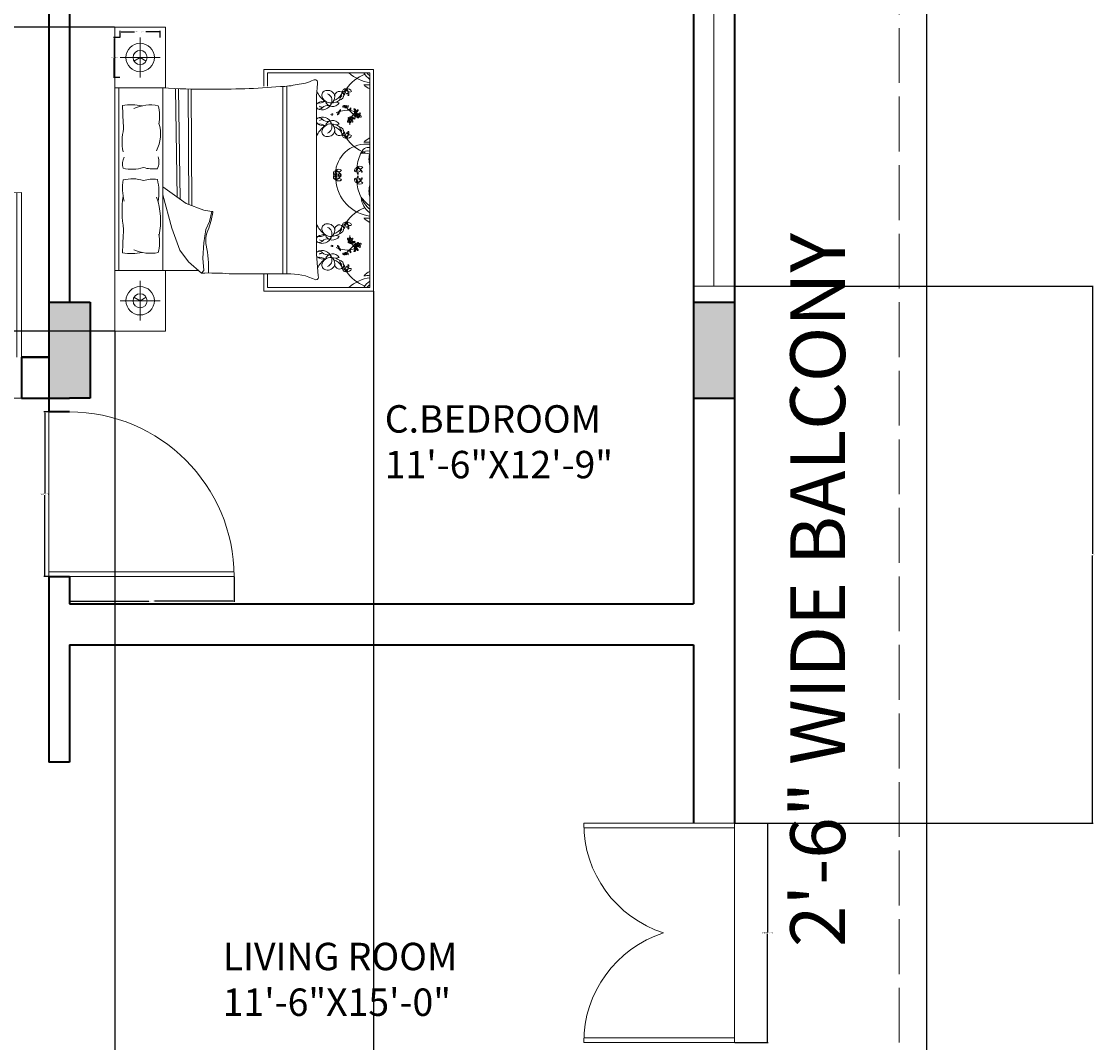
# Model space of a CAD drawing. Units: inches. Extents: x -36 to 401, y -686 to 73.
# Tile 14 of 15: x 167 to 401, y -319 to -96. Entities that reach past the tile are written whole.
import ezdxf

# ---------------------------------------------------------------- set-up
doc = ezdxf.new("R2010")
doc.units = ezdxf.units.IN
doc.header["$MEASUREMENT"] = 0
doc.linetypes.add('ACAD_ISO02W100', pattern=[15, 12, -3])
for name, color, linetype, lineweight in [('A-ANNO-DIMS', 2, 'Continuous', 18), ('A-AREA-IDEN', 7, 'Continuous', 18), ('A-COLS', 7, 'Continuous', 40), ('A-COLS-PATT', 22, 'Continuous', 13), ('A-DOOR', 3, 'Continuous', 18), ('A-FLOR-OVHD', 8, 'ACAD_ISO02W100', 18), ('A-FURN', 8, 'Continuous', 13), ('A-GLAZ', 4, 'Continuous', 18), ('A-WALL', 7, 'Continuous', 35), ('C-PROP', 7, 'Continuous', 25)]:
    doc.layers.add(name, color=color, linetype=linetype, lineweight=lineweight)
doc.styles.get("Standard").update_dxf_attribs({"font": 'arial.ttf'})
doc.dimstyles.get("Standard").update_dxf_attribs({"dimtxt": 0.18, "dimasz": 0.18, "dimexe": 0.18, "dimexo": 0.0625, "dimgap": 0.09, "dimtad": 0, "dimtih": 1, "dimtoh": 1, "dimdec": 0, "dimzin": 0, "dimdsep": 46, "dimlunit": 3, "dimtxsty": 'Standard', "dimcen": 0.09, "dimadec": 0, "dimazin": 0, "dimtfac": 1, "dimtdec": 0, "dimtofl": 0, "dimtmove": 0, "dimatfit": 3, "dimfxl": 1, "dimtolj": 1, "dimtzin": 0, "dimarcsym": 0})

# ---------------------------------------------------------------- blocks, each defined once
blk = doc.blocks.new('WIN-60IN')
for p, q in [((0, 9), (60, 9)), ((0, 0), (0, 9)), ((60, 9), (60, 0)), ((0, 4.5), (60, 4.5)), ((60, 0), (0, 0))]:
    blk.add_line(p, q)
blk = doc.blocks.new('DOOR-SWING-36IN')
for p, q in [((-1, 0), (-1, 36)), ((0, 0), (0, 36))]:
    blk.add_line(p, q)
blk.add_arc((0, 0), 36, 90, 180)
blk = doc.blocks.new('DOOR-PAIR-48IN')
for p, q in [((0, 48), (-24, 48)), ((0, 47), (-24, 47)), ((9, 48), (0, 48)), ((9, 47), (0, 47)), ((0, 1), (-24, 1)), ((0, 0), (-24, 0)), ((0, 1), (9, 1)), ((0, 0), (9, 0))]:
    blk.add_line(p, q)
for centre, start, end in [((1.23, 48), 180, 252.0547), ((1.23, 0), 107.9453, 180)]:
    blk.add_arc(centre, 25.23, start, end)
blk = doc.blocks.new('LAMP-BEDSIDE-SMALL')
for p, q in [((4.35, 0), (4.35, 8.7)), ((8.7, 4.35), (0, 4.35))]:
    blk.add_line(p, q)
for points in [[(4.35, 4.35), (3, 3.57)], [(4.35, 4.35), (5.69, 3.57)]]:
    blk.add_lwpolyline(points)
for radius in [3.11, 1.55]:
    blk.add_circle((4.35, 4.35), radius)
blk = doc.blocks.new('*D41')
at = {"layer": 'A-ANNO-DIMS', "color": 0, "lineweight": -2, "transparency": 16777216}
for p, q in [((177.13, -181.21), (171.61, -181.21)), ((171.79, -181.39), (171.79, -199.03)), ((171.79, -217.03), (171.79, -199.39)), ((177.13, -217.21), (171.61, -217.21))]:
    blk.add_line(p, q, dxfattribs=at)
at = {"layer": 'A-ANNO-DIMS', "color": 0, "transparency": 16777216}
for points in [[(171.76, -181.39), (171.82, -181.39), (171.79, -181.21)], [(171.76, -217.03), (171.82, -217.03), (171.79, -217.21)]]:
    blk.add_solid(points, dxfattribs=at)
at = {"layer": 'Defpoints', "color": 0, "transparency": 16777216}
for p in [(177.19, -181.21), (171.79, -217.21), (177.19, -217.21)]:
    blk.add_point(p, dxfattribs=at)
at = {"layer": 'A-ANNO-DIMS', "color": 0, "transparency": 16777216, "insert": (171.79, -199.21), "char_height": 0.18, "attachment_point": 5}
blk.add_mtext('\\A1;DOOR 3\'-0" TYP.', dxfattribs=at)
blk = doc.blocks.new('*D42')
at = {"layer": 'A-ANNO-DIMS', "color": 0, "lineweight": -2, "transparency": 16777216}
for p, q in [((177.19, -217.27), (177.19, -222.79)), ((213.19, -217.27), (213.19, -222.79)), ((177.37, -222.61), (194.55, -222.61)), ((213.01, -222.61), (195.83, -222.61))]:
    blk.add_line(p, q, dxfattribs=at)
at = {"layer": 'A-ANNO-DIMS', "color": 0, "transparency": 16777216}
for points in [[(177.37, -222.58), (177.37, -222.64), (177.19, -222.61)], [(213.01, -222.58), (213.01, -222.64), (213.19, -222.61)]]:
    blk.add_solid(points, dxfattribs=at)
at = {"layer": 'Defpoints', "color": 0, "transparency": 16777216}
for p in [(177.19, -217.21), (213.19, -217.21), (213.19, -222.61)]:
    blk.add_point(p, dxfattribs=at)
at = {"layer": 'A-ANNO-DIMS', "color": 0, "transparency": 16777216, "insert": (195.19, -222.61), "char_height": 0.18, "attachment_point": 5}
blk.add_mtext('\\A1;3\'-0" TYP.', dxfattribs=at)
blk = doc.blocks.new('*D45')
at = {"layer": 'A-ANNO-DIMS', "color": 0, "lineweight": -2, "transparency": 16777216}
for p, q in [((322.75, -271.21), (330.07, -271.21)), ((329.89, -271.39), (329.89, -295.03)), ((329.89, -319.03), (329.89, -295.39)), ((322.75, -319.21), (330.07, -319.21))]:
    blk.add_line(p, q, dxfattribs=at)
at = {"layer": 'A-ANNO-DIMS', "color": 0, "transparency": 16777216}
for points in [[(329.86, -271.39), (329.92, -271.39), (329.89, -271.21)], [(329.86, -319.03), (329.92, -319.03), (329.89, -319.21)]]:
    blk.add_solid(points, dxfattribs=at)
at = {"layer": 'Defpoints', "color": 0, "transparency": 16777216}
for p in [(322.69, -271.21), (329.89, -271.21), (322.69, -319.21)]:
    blk.add_point(p, dxfattribs=at)
at = {"layer": 'A-ANNO-DIMS', "color": 0, "transparency": 16777216, "insert": (329.89, -295.21), "char_height": 0.18, "attachment_point": 5}
blk.add_mtext('\\A1;DOOR PAIR 4\'-0" TYP.', dxfattribs=at)
blk = doc.blocks.new('*D59')
at = {"layer": 'A-ANNO-DIMS', "color": 0, "lineweight": -2, "transparency": 16777216}
for p, q in [((188.3, -99.23), (188.3, -97.81)), ((188.48, -97.99), (191.43, -97.99)), ((196.82, -97.99), (193.87, -97.99)), ((197, -99.23), (197, -97.81))]:
    blk.add_line(p, q, dxfattribs=at)
at = {"layer": 'A-ANNO-DIMS', "color": 0, "transparency": 16777216}
for points in [[(188.48, -97.96), (188.48, -98.02), (188.3, -97.99)], [(196.82, -97.96), (196.82, -98.02), (197, -97.99)]]:
    blk.add_solid(points, dxfattribs=at)
at = {"layer": 'Defpoints', "color": 0, "transparency": 16777216}
for p in [(197, -97.99), (188.3, -99.29), (197, -99.29)]:
    blk.add_point(p, dxfattribs=at)
at = {"layer": 'A-ANNO-DIMS', "color": 0, "transparency": 16777216, "insert": (192.65, -97.99), "char_height": 0.18, "attachment_point": 5}
blk.add_mtext('\\A1;LAMP 0\'-8 1/2" TYP.', dxfattribs=at)
blk = doc.blocks.new('*D60')
at = {"layer": 'A-ANNO-DIMS', "color": 0, "lineweight": -2, "transparency": 16777216}
for p, q in [((188.24, -99.29), (186.82, -99.29)), ((187, -99.47), (187, -103.46)), ((187, -107.81), (187, -103.82)), ((188.24, -107.99), (186.82, -107.99))]:
    blk.add_line(p, q, dxfattribs=at)
at = {"layer": 'A-ANNO-DIMS', "color": 0, "transparency": 16777216}
for points in [[(186.97, -99.47), (187.03, -99.47), (187, -99.29)], [(186.97, -107.81), (187.03, -107.81), (187, -107.99)]]:
    blk.add_solid(points, dxfattribs=at)
at = {"layer": 'Defpoints', "color": 0, "transparency": 16777216}
for p in [(187, -99.29), (188.3, -99.29), (188.3, -107.99)]:
    blk.add_point(p, dxfattribs=at)
at = {"layer": 'A-ANNO-DIMS', "color": 0, "transparency": 16777216, "insert": (187, -103.64), "char_height": 0.18, "attachment_point": 5}
blk.add_mtext('\\A1;0\'-8 1/2" TYP.', dxfattribs=at)
blk = doc.blocks.new('*D71')
at = {"layer": 'A-ANNO-DIMS', "color": 0, "lineweight": -2, "transparency": 16777216}
for p, q in [((322.75, -153.68), (401.17, -153.68)), ((400.99, -153.86), (400.99, -212.26)), ((400.99, -271.03), (400.99, -212.63)), ((322.75, -271.21), (401.17, -271.21))]:
    blk.add_line(p, q, dxfattribs=at)
at = {"layer": 'A-ANNO-DIMS', "color": 0, "transparency": 16777216}
for points in [[(400.96, -153.86), (401.02, -153.86), (400.99, -153.68)], [(400.96, -271.03), (401.02, -271.03), (400.99, -271.21)]]:
    blk.add_solid(points, dxfattribs=at)
at = {"layer": 'Defpoints', "color": 0, "transparency": 16777216}
for p in [(322.69, -153.68), (322.69, -271.21), (400.99, -271.21)]:
    blk.add_point(p, dxfattribs=at)
at = {"layer": 'A-ANNO-DIMS', "color": 0, "transparency": 16777216, "insert": (400.99, -212.44), "char_height": 0.18, "attachment_point": 5}
blk.add_mtext('\\A1;9\'-9 1/2"', dxfattribs=at)
blk = doc.blocks.new('*D87')
at = {"layer": 'A-ANNO-DIMS', "color": 0, "lineweight": -2, "transparency": 16777216}
for p, q in [((243.7, -154.81), (243.7, -685.69)), ((187.11, -163.6), (187.11, -685.69)), ((187.29, -685.51), (214.86, -685.51)), ((243.52, -685.51), (215.95, -685.51))]:
    blk.add_line(p, q, dxfattribs=at)
at = {"layer": 'A-ANNO-DIMS', "color": 0, "transparency": 16777216}
for points in [[(187.29, -685.48), (187.29, -685.54), (187.11, -685.51)], [(243.52, -685.48), (243.52, -685.54), (243.7, -685.51)]]:
    blk.add_solid(points, dxfattribs=at)
at = {"layer": 'Defpoints', "color": 0, "transparency": 16777216}
for p in [(243.7, -154.75), (187.11, -163.53), (243.7, -685.51)]:
    blk.add_point(p, dxfattribs=at)
at = {"layer": 'A-ANNO-DIMS', "color": 0, "transparency": 16777216, "insert": (215.4, -685.51), "char_height": 0.18, "attachment_point": 5}
blk.add_mtext('\\A1;4\'-8 1/2"', dxfattribs=at)
blk = doc.blocks.new('*D88')
at = {"layer": 'A-ANNO-DIMS', "color": 0, "lineweight": -2, "transparency": 16777216}
for p, q in [((187.04, -96.98), (-34.79, -96.98)), ((-34.61, -97.16), (-34.61, -130.08)), ((-34.61, -163.35), (-34.61, -130.44)), ((187.04, -163.53), (-34.79, -163.53))]:
    blk.add_line(p, q, dxfattribs=at)
at = {"layer": 'A-ANNO-DIMS', "color": 0, "transparency": 16777216}
for points in [[(-34.64, -97.16), (-34.58, -97.16), (-34.61, -96.98)], [(-34.64, -163.35), (-34.58, -163.35), (-34.61, -163.53)]]:
    blk.add_solid(points, dxfattribs=at)
at = {"layer": 'Defpoints', "color": 0, "transparency": 16777216}
for p in [(187.11, -96.98), (-34.61, -163.53), (187.11, -163.53)]:
    blk.add_point(p, dxfattribs=at)
at = {"layer": 'A-ANNO-DIMS', "color": 0, "transparency": 16777216, "insert": (-34.61, -130.26), "char_height": 0.18, "attachment_point": 5}
blk.add_mtext('\\A1;5\'-6 1/2"', dxfattribs=at)

msp = doc.modelspace()

# ---------------------------------------------------------------- hatches: boundary and pattern name
at = {"layer": 'A-COLS-PATT'}
h = msp.add_hatch(color=256, dxfattribs=at)
h.dxf.hatch_style = 1
h.paths.add_polyline_path([(34.69, 7.79), (25.69, 7.79), (25.69, -13.21), (34.69, -13.21)])
h.paths.add_polyline_path([(172.69, -13.21), (177.19, -13.21), (181.69, -13.21), (181.69, 7.79), (172.69, 7.79)])
h.paths.add_polyline_path([(322.69, 7.79), (313.69, 7.79), (313.69, -13.21), (322.69, -13.21)])
h.paths.add_polyline_path([(322.69, -157.21), (313.69, -157.21), (313.69, -178.21), (322.69, -178.21)])
h.paths.add_polyline_path([(172.69, -178.21), (177.19, -178.21), (181.69, -178.21), (181.69, -157.21), (177.19, -157.21), (172.69, -157.21)])
h.paths.add_polyline_path([(25.69, -178.21), (34.69, -178.21), (34.69, -157.21), (25.69, -157.21)])
h.paths.add_polyline_path([(34.69, -325.21), (25.69, -325.21), (25.69, -346.21), (34.69, -346.21)])
h.paths.add_polyline_path([(181.69, -325.21), (177.19, -325.21), (172.69, -325.21), (172.69, -346.21), (177.19, -346.21), (181.69, -346.21)])
h.paths.add_polyline_path([(322.69, -325.21), (313.69, -325.21), (313.69, -346.21), (322.69, -346.21)])
h.paths.add_polyline_path([(364.69, -451.21), (358.69, -451.21), (358.69, -472.21), (364.69, -472.21)])
h.paths.add_polyline_path([(181.69, -451.21), (177.19, -451.21), (172.69, -451.21), (172.69, -472.21), (177.19, -472.21), (181.69, -472.21)])
h.paths.add_polyline_path([(25.69, -472.21), (34.69, -472.21), (34.69, -451.21), (25.69, -451.21)])

# ---------------------------------------------------------------- linework, layer by layer
at = {"layer": 'A-COLS'}
for p, q in [((172.69, -157.21), (177.19, -157.21)), ((177.19, -157.21), (181.69, -157.21)), ((181.69, -157.21), (181.69, -178.21)), ((313.69, -157.21), (322.69, -157.21)), ((181.69, -178.21), (177.19, -178.21)), ((313.69, -178.21), (322.69, -178.21))]:
    msp.add_line(p, q, dxfattribs=at)
at = {"layer": 'A-DOOR'}
for p, q in [((130.69, -178.21), (166.69, -178.21)), ((172.69, -217.21), (172.69, -181.21)), ((172.69, -216.21), (177.19, -216.21)), ((322.69, -271.21), (322.69, -319.21))]:
    msp.add_line(p, q, dxfattribs=at)
at = {"layer": 'A-FLOR-OVHD'}
msp.add_line((358.69, 7.79), (358.69, -559.77), dxfattribs=at)
at = {"layer": 'A-FURN'}
for p, q in [((187.11, -163.53), (187.11, -96.98)), ((219.73, -109.92), (219.73, -106.23)), ((219.73, -106.23), (243.7, -106.23)), ((220.5, -107), (220.5, -109.94)), ((242.93, -107), (220.5, -107)), ((242.93, -153.98), (242.93, -107)), ((243.7, -106.23), (243.7, -154.75)), ((187.96, -110.29), (187.96, -150.22)), ((197.62, -150.22), (197.62, -110.29)), ((223.88, -109.99), (223.88, -150.99)), ((224.71, -109.93), (224.71, -150.99)), ((200.39, -110.47), (200.72, -134.17)), ((201.07, -110.5), (201.41, -134.66)), ((203.17, -110.53), (203.27, -135.8)), ((203.85, -110.53), (203.95, -136.07)), ((236.18, -113.56), (235.43, -113.42)), ((231.25, -116.75), (231.25, -143.77)), ((236.18, -118.21), (235.43, -118.36)), ((197.62, -131.94), (202.7, -135.59)), ((199.6, -140.98), (197.62, -133.72)), ((202.7, -135.59), (206.61, -137.07)), ((206.61, -137.07), (208.36, -137.34)), ((208.36, -137.34), (207.82, -139.5)), ((207.82, -139.5), (207.01, -141.25)), ((201.35, -145.83), (199.6, -140.98)), ((207.01, -141.25), (206.61, -144.22)), ((236.18, -142.77), (235.43, -142.62)), ((206.61, -144.22), (206.34, -147.59)), ((203.24, -148.39), (201.35, -145.83)), ((206.34, -147.59), (206.61, -150.28)), ((236.18, -147.42), (235.43, -147.57)), ((187.11, -150.22), (205.37, -150.22)), ((206.07, -150.82), (203.24, -148.39)), ((206.61, -150.28), (206.07, -150.82)), ((219.73, -154.75), (219.73, -150.99)), ((220.5, -150.99), (220.5, -153.98)), ((243.7, -154.75), (219.73, -154.75)), ((220.5, -153.98), (242.93, -153.98))]:
    msp.add_line(p, q, dxfattribs=at)
for points in [[(187.11, -110.29), (198.2, -110.29), (198.2, -96.98), (187.11, -96.98)], [(198.2, -150.22), (198.2, -163.53), (187.11, -163.53)]]:
    msp.add_lwpolyline(points, dxfattribs=at)
for points in [[(223.36, -110.01, 0.056112), (227.02, -109.53, 0.095341), (230.54, -108.59)], [(188.77, -114.12, -0.074897), (193.11, -114.2, 0.472817)], [(193.36, -127.73, -0.14099), (188.92, -127.86, -0.235245)], [(193.36, -130.57, 0.14099), (188.92, -130.44, 0.235245)], [(188.77, -146.4, 0.074897), (193.11, -146.32, -0.472817)], [(212.16, -150.96, 0.001242), (224.79, -150.99, -0.127202), (231.08, -152.33)]]:
    msp.add_lwpolyline(points, format="xyb", dxfattribs=at)
for centre in [(238.6, -117.41), (240.38, -116.3), (238.6, -143.58), (240.38, -144.68)]:
    msp.add_circle(centre, 0.169, dxfattribs=at)
for centre, radius, start, end in [((244.96, -115.4), 8.69, 111.4092, 145.6135), ((244.1, -100.53), 8.69, 228.1144, 262.255), ((245.27, -104.89), 4.23, 209.8884, 236.5383), ((246.06, -103.37), 5.28, 223.5186, 233.6964), ((205.76, 9.01), 119.58, 266.1, 270.9282), ((210.1, 45.41), 155.98, 269.1145, 274.8735), ((230.88, -109.1), 0.607, 336.5219, 123.8264), ((295.97, -114.71), 64.76, 175.2402, 181.8035), ((244.29, -107.27), 3.53, 221.0454, 247.4453), ((242.39, -97.59), 12.02, 266.3481, 272.5919), ((235.93, -109.01), 5.04, 203.6453, 236.3329), ((233.52, -111.95), 1.12, 88.9462, 185.5144), ((234.35, -111.6), 2, 193.079, 274.7067), ((233.68, -112.41), 1.59, 7.1143, 95.0551), ((233.07, -113.03), 1.54, 338.5779, 68.4181), ((233.32, -112.13), 1.93, 305.9599, 357.6409), ((234.04, -110.06), 3.14, 288.2955, 328.7386), ((236.24, -112.04), 0.999, 19.1312, 189.736), ((235.94, -111.8), 1.25, 285.6955, 4.031), ((237.6, -113.14), 1.33, 128.4175, 173.8338), ((237.32, -111.83), 0.612, 126.7319, 206.0245), ((237.62, -111.19), 0.72, 76.272, 177.0484), ((236.52, -109.72), 1.48, 284.7031, 328.6173), ((238.59, -111.61), 1.37, 125.7657, 194.5347), ((231.85, -109.18), 6.08, 332.8176, 347.4827), ((238, -111.44), 0.964, 20.9613, 102.2885), ((238.52, -110.47), 0.726, 181.7131, 301.5367), ((236.14, -111.94), 2.2, 2.0648, 41.1598), ((237.46, -111.12), 0.711, 316.2238, 62.3173), ((237.87, -111.54), 0.0567, 20.2667, 316.2271), ((238.17, -111.85), 0.0524, 52.0591, 168.5166), ((238.22, -111.87), 0.108, 168.5166, 2.0648), ((-444.57, -150.8), 634.39, 2.85022, 3.31479), ((194.86, -122.6), 8.58, 78.2417, 114.8684), ((187.99, -116.49), 8.92, 348.9631, 14.8961), ((231.98, -114.27), 0.801, 127.675, 162.5814), ((231.98, -114.27), 0.801, 196.6343, 225.5483), ((231.74, -110.86), 2.76, 259.249, 301.1782), ((232.46, -112.99), 2.12, 240.8249, 340.7178), ((231.82, -113.93), 0.996, 246.1646, 318.4347), ((232.94, -115.76), 2.57, 85.2696, 124.215), ((232.84, -112.67), 1.91, 240.0851, 262.564), ((233.59, -115.5), 1.36, 74.8529, 138.4347), ((234.75, -112.74), 1.65, 196.8663, 330.0915), ((234.05, -113.78), 0.413, 254.8529, 12.6959), ((232.94, -115.76), 2.57, 53.6555, 57.2989), ((234.29, -110.03), 3.57, 273.4924, 303.7117), ((236.66, -115.34), 0.349, 115.5379, 168.6744), ((235.48, -114.84), 1.05, 329.344, 349.7412), ((234.64, -115.08), 1.88, 352.8698, 1.6736), ((237.12, -114.41), 0.131, 125.0752, 284.7644), ((237.33, -114.36), 0.283, 127.3642, 168.4363), ((237.1, -114.13), 0.408, 277.4968, 341.2737), ((237.43, -114.32), 0.162, 88.1325, 178.8919), ((237.75, -114.49), 0.35, 136.3462, 189.6513), ((237.55, -114.53), 0.146, 189.6513, 312.3208), ((237.59, -114.12), 0.169, 183.2768, 356.7232), ((238.12, -114.42), 0.555, 164.2829, 186.9148), ((237.46, -114.43), 0.277, 312.3208, 40.2111), ((238.05, -114.12), 0.394, 201.6382, 274.947), ((237.53, -114.65), 0.515, 42.3896, 66.5724), ((242.72, -110.58), 6.32, 217.9541, 226.8459), ((237.9, -114.35), 0.28, 10.9597, 52.2379), ((238.07, -114.38), 0.13, 274.947, 37.5263), ((238.51, -115.12), 0.136, 112.5583, 214.2343), ((238.42, -114.87), 0.319, 265.7131, 351.6568), ((238.14, -114.7), 0.558, 297.3659, 329.344), ((237.72, -114.22), 1.07, 313.6929, 321.7899), ((238.9, -114.95), 0.349, 115.5379, 168.6744), ((237.72, -114.44), 1.05, 329.344, 349.7412), ((236.88, -114.69), 1.88, 352.8698, 1.6736), ((239.52, -115.07), 0.189, 33.0979, 123.1364), ((235.35, -117.73), 4.95, 31.1156, 34.8118), ((239.24, -115.39), 0.512, 2.3172, 70.5201), ((239.44, -115.33), 0.441, 352.6008, 57.1845), ((231.98, -117.5), 0.801, 134.4517, 156.7144), ((232.46, -118.78), 2.12, 19.2822, 119.1751), ((231.82, -117.84), 0.996, 41.5653, 113.8354), ((232.84, -119.1), 1.91, 97.436, 119.9149), ((233.59, -116.28), 1.36, 221.5653, 285.1471), ((234.6, -116.06), 0.209, 169.5864, 349.5616), ((234.68, -116.08), 0.128, 349.5616, 167.2949), ((238.03, -120.69), 5.51, 110.1059, 116.9968), ((236.18, -116.15), 0.349, 129.5056, 182.6421), ((235.18, -115.34), 1.05, 308.4388, 328.836), ((235, -114.49), 1.88, 296.5064, 305.3102), ((234.98, -115.45), 1.07, 336.3901, 344.4871), ((236.15, -115.72), 0.136, 83.9457, 185.6216), ((235.6, -115.6), 0.558, 328.836, 0.8141), ((235.89, -115.76), 0.319, 306.5232, 32.4668), ((236.27, -115.51), 0.136, 112.5583, 214.2343), ((236.18, -115.27), 0.319, 265.7131, 351.6568), ((235.9, -115.09), 0.558, 297.3659, 329.344), ((235.48, -114.61), 1.07, 313.6929, 321.7899), ((238.03, -120.69), 5.51, 86.1723, 106.4158), ((238.33, -117.64), 0.283, 93.635, 168.4363), ((238.34, -116.11), 0.773, 253.6301, 325.4631), ((238.56, -117.18), 0.546, 82.0748, 142.6895), ((238.5, -116.43), 0.561, 228.342, 274.9894), ((238.3, -117.19), 0.166, 138.2946, 276.2474), ((238.36, -117.22), 0.231, 358.5719, 143.8954), ((238.49, -117.04), 0.233, 208.8493, 269.9355), ((238.3, -117.09), 0.267, 274.2123, 318.1587), ((238.17, -117.95), 2.76, 60.7959, 85.244), ((232.29, -121.92), 9.09, 37.8256, 47.7588), ((238.52, -116.52), 0.47, 273.8774, 357.1501), ((239.11, -117.36), 0.534, 121.9501, 165.2442), ((238.7, -116.19), 0.455, 262.0748, 308.2393), ((238.74, -117.16), 0.112, 262.868, 7.094), ((238.73, -117.06), 0.334, 278.5614, 22.5914), ((238.91, -117.64), 0.28, 10.9597, 118.7804), ((241.84, -118.23), 3.31, 156.1523, 156.9499), ((238.91, -117.05), 0.168, 44.3732, 121.9501), ((239.43, -116.66), 0.47, 181.4625, 249.4747), ((239.35, -116.29), 0.455, 215.1128, 261.2773), ((239.72, -116.31), 0.773, 197.889, 269.722), ((241.84, -118.23), 3.31, 130.182, 149.456), ((239.47, -116.57), 0.561, 248.3627, 295.0101), ((239.2, -117.28), 0.546, 20.6625, 81.2773), ((240.02, -116.34), 0.546, 139.3812, 199.9959), ((239, -115.95), 0.773, 310.9365, 22.7695), ((239.35, -115.99), 0.561, 285.6484, 332.2957), ((239.66, -115.52), 0.148, 135.7354, 318.1297), ((239.42, -115.28), 0.196, 315.7354, 31.1156), ((239.26, -115.69), 0.455, 319.3812, 5.5456), ((239.78, -115.52), 0.148, 68.2452, 250.6395), ((241.01, -118.29), 2.95, 111.7087, 116.2181), ((238.17, -117.95), 2.76, 47.5083, 55.9967), ((239.86, -115.23), 0.441, 252.8042, 349.6943), ((239.44, -116.02), 0.47, 331.1838, 51.6792), ((239.92, -116.58), 0.131, 125.0752, 284.7644), ((239.9, -115.2), 0.196, 248.2452, 323.6254), ((240.12, -116.53), 0.283, 93.635, 168.4363), ((239.73, -115.08), 0.512, 291.7087, 3.0299), ((240.08, -116.09), 0.166, 138.2946, 276.2474), ((239.9, -116.31), 0.408, 277.4968, 341.2737), ((240.15, -116.11), 0.231, 358.5719, 143.8954), ((236.07, -112.38), 4.95, 323.6254, 327.3216), ((240.22, -116.5), 0.162, 88.1325, 178.8919), ((240.28, -115.93), 0.233, 208.8493, 269.9355), ((240.08, -115.98), 0.267, 274.2123, 318.1587), ((240.55, -116.67), 0.35, 136.3462, 189.6513), ((240.35, -116.7), 0.146, 189.6513, 312.3208), ((240.14, -115.21), 0.189, 325.6077, 55.6462), ((240.91, -116.6), 0.555, 164.2829, 186.9148), ((240.89, -116.25), 0.534, 121.9501, 165.2442), ((240.26, -116.61), 0.277, 312.3208, 40.2111), ((240.84, -116.29), 0.394, 201.6382, 274.947), ((240.53, -116.05), 0.112, 262.868, 7.094), ((240.32, -116.83), 0.515, 42.3896, 66.5724), ((240.51, -115.95), 0.334, 278.5614, 22.5914), ((240.7, -116.53), 0.28, 10.9597, 118.7804), ((240.7, -115.94), 0.168, 44.3732, 121.9501), ((240.87, -116.56), 0.13, 274.947, 37.5263), ((200.41, -122.02), 11.7, 166.3427, 191.1841), ((188.64, -120.34), 8.47, 333.8761, 16.1746), ((231.98, -117.5), 0.801, 203.2856, 232.325), ((231.74, -120.92), 2.76, 58.8218, 100.2867), ((235.93, -122.76), 5.04, 123.6671, 158.5059), ((232.94, -116.01), 2.57, 235.785, 274.7304), ((233.52, -119.83), 1.12, 174.4856, 271.0538), ((234.35, -120.18), 2, 85.2933, 166.921), ((234.75, -119.04), 1.65, 29.9085, 163.1337), ((233.68, -119.37), 1.59, 264.9449, 352.8857), ((233.07, -118.74), 1.54, 291.5819, 21.4221), ((234.05, -117.99), 0.413, 347.3041, 105.1471), ((232.94, -116.01), 2.57, 302.7011, 306.3445), ((233.32, -119.65), 1.93, 2.3591, 54.0401), ((234.29, -121.75), 3.57, 56.2883, 86.5076), ((234.04, -121.72), 3.14, 31.2614, 71.7045), ((236.24, -119.74), 0.999, 170.264, 340.8688), ((237.6, -118.63), 1.33, 186.1662, 231.5825), ((235.94, -119.98), 1.25, 355.969, 74.3045), ((237.32, -119.94), 0.612, 153.9755, 233.2681), ((238.13, -117.69), 0.131, 125.0752, 284.7644), ((238.11, -117.41), 0.408, 277.4968, 341.2737), ((238.44, -117.6), 0.162, 88.1325, 178.8919), ((238.76, -117.78), 0.35, 136.3462, 189.6513), ((238.56, -117.81), 0.146, 189.6513, 312.3208), ((241.84, -118.23), 3.31, 175.2415, 182.8929), ((239.13, -117.71), 0.555, 164.2829, 186.9148), ((238.47, -117.71), 0.277, 312.3208, 40.2111), ((239.06, -117.4), 0.394, 201.6382, 274.947), ((238.54, -117.94), 0.515, 42.3896, 66.5724), ((239.08, -117.66), 0.13, 274.947, 37.5263), ((237.62, -120.58), 0.72, 182.9516, 283.728), ((236.52, -122.05), 1.48, 31.3827, 75.2969), ((238.59, -120.17), 1.37, 165.4653, 234.2343), ((231.85, -122.6), 6.08, 12.5173, 27.1824), ((236.14, -119.83), 2.2, 318.8402, 357.9352), ((237.46, -120.65), 0.711, 297.6827, 43.7762), ((238.52, -121.3), 0.726, 58.4633, 178.2869), ((238, -120.34), 0.964, 257.7115, 339.0387), ((244.96, -116.37), 8.69, 214.3865, 248.5908), ((237.91, -120.23), 0.094, 43.7762, 339.7183), ((238.22, -119.91), 0.108, 357.9352, 191.4834), ((238.17, -119.92), 0.0524, 191.4834, 307.9409), ((244.29, -124.51), 3.53, 112.5547, 138.9546), ((242.1, -129.3), 6.73, 82.8636, 171.8197), ((248.76, -128.36), 8.69, 152.5854, 175.5377), ((242.56, -124.86), 1.56, 76.3898, 169.0739), ((242.35, -126.04), 1.97, 72.8609, 131.9049), ((242.39, -134.19), 12.02, 87.4081, 93.6519), ((192.08, -126.95), 3.29, 153.3437, 196.1026), ((193.23, -126.5), 3.53, 335.0183, 18.5407), ((241.48, -128.43), 3.89, 68.117, 96.6195), ((247.5, -125.93), 4.78, 162.9798, 196.4569), ((195.58, -119.88), 8.15, 254.1707, 275.9871), ((235.64, -129.04), 0.72, 106.1963, 206.9726), ((233.95, -128.31), 1.48, 314.6273, 358.5415), ((236.69, -128.91), 1.37, 155.6899, 224.4589), ((236.69, -129.85), 1.37, 135.5411, 204.3101), ((236.09, -129.06), 0.964, 50.8855, 132.2127), ((236.06, -127.97), 0.726, 211.6373, 331.4609), ((235.47, -129.06), 0.711, 346.148, 92.2415), ((234.73, -130.43), 2.2, 31.989, 71.0841), ((229.64, -130.17), 6.08, 2.7418, 17.407), ((229.64, -128.6), 6.08, 342.593, 357.2582), ((240.29, -128.37), 0.72, 106.1963, 206.9726), ((238.61, -127.64), 1.48, 314.6273, 358.5415), ((241.35, -128.25), 1.37, 155.6899, 224.4589), ((240.74, -128.4), 0.964, 50.8855, 132.2127), ((240.71, -127.3), 0.726, 211.6373, 331.4609), ((239.38, -129.76), 2.2, 31.989, 71.0841), ((234.29, -129.5), 6.08, 2.7418, 17.407), ((240.12, -128.39), 0.711, 346.148, 92.2415), ((240.68, -128.55), 0.0567, 50.1909, 346.0209), ((241.15, -128.65), 0.108, 198.4408, 31.989), ((241.1, -128.67), 0.0524, 81.9833, 198.4408), ((249.96, -127.82), 7.07, 174.3643, 175.6213), ((254.8, -131.54), 12.63, 160.0972, 160.2783), ((200.65, -132.19), 11.86, 171.5249, 193.96), ((195.58, -138.42), 8.15, 84.0129, 105.8293), ((185.02, -133.07), 11.74, 349.8617, 13.6238), ((235.64, -129.73), 0.72, 153.0274, 253.8037), ((233.95, -130.46), 1.48, 1.4585, 45.3727), ((234.73, -128.34), 2.2, 288.9159, 328.011), ((235.47, -129.71), 0.711, 267.7585, 13.852), ((236.06, -130.8), 0.726, 28.5391, 148.3627), ((236.09, -129.7), 0.964, 227.7873, 309.1145), ((244.1, -129.74), 8.69, 184.4623, 262.255), ((236.03, -129.21), 0.0567, 50.1909, 346.0209), ((236.07, -129.56), 0.094, 13.852, 309.9245), ((236.45, -129.34), 0.0524, 81.9833, 198.4408), ((236.45, -129.43), 0.0524, 161.5592, 278.0167), ((236.5, -129.32), 0.108, 198.4408, 31.989), ((236.5, -129.45), 0.108, 328.011, 161.5592), ((240.29, -130.39), 0.72, 153.0274, 253.8037), ((238.61, -131.12), 1.48, 1.4585, 45.3727), ((241.35, -130.52), 1.37, 135.5411, 204.3101), ((234.29, -129.26), 6.08, 342.593, 357.2582), ((239.38, -129), 2.2, 288.9159, 328.011), ((240.12, -130.37), 0.711, 267.7585, 13.852), ((240.71, -131.46), 0.726, 28.5391, 148.3627), ((240.74, -130.37), 0.964, 227.7873, 309.1145), ((248.76, -130.41), 8.69, 184.4623, 207.4146), ((240.72, -130.23), 0.094, 13.852, 309.9245), ((241.15, -130.11), 0.108, 328.011, 161.5592), ((241.1, -130.09), 0.0524, 161.5592, 278.0167), ((247.5, -132.84), 4.78, 163.5431, 197.0202), ((249.96, -130.94), 7.07, 184.3787, 185.6357), ((254.8, -127.22), 12.63, 199.7217, 199.9028), ((212.85, -137.28), 24.14, 172.2196, 189.497), ((181.65, -139.33), 15.47, 348.0397, 19.2615), ((245.27, -134.1), 4.23, 181.272, 236.5383), ((247.54, -129.8), 7.85, 214.0123, 234.053), ((246.06, -132.58), 5.28, 197.8504, 233.6964), ((183.21, -132.72), 25.81, 340.1194, 349.3383), ((208.41, -137.49), 0.161, 358.8623, 109.7536), ((244.96, -144.61), 8.69, 111.4092, 145.6135), ((235.93, -138.22), 5.04, 201.4941, 236.3329), ((233.52, -141.15), 1.12, 88.9462, 185.5144), ((233.68, -141.61), 1.59, 7.1143, 95.0551), ((233.07, -142.24), 1.54, 338.5779, 68.4181), ((236.24, -141.25), 0.999, 19.1312, 189.736), ((237.32, -141.04), 0.612, 126.7319, 206.0245), ((237.62, -140.4), 0.72, 76.272, 177.0484), ((236.52, -138.93), 1.48, 284.7031, 328.6173), ((238.59, -140.82), 1.37, 125.7657, 194.5347), ((231.85, -138.38), 6.08, 332.8176, 347.4827), ((238, -140.64), 0.964, 20.9613, 102.2885), ((237.46, -140.33), 0.711, 316.2238, 62.3173), ((236.14, -141.15), 2.2, 2.0648, 41.1598), ((238.52, -139.68), 0.726, 181.7131, 301.5367), ((237.87, -140.75), 0.0567, 20.2667, 316.2271), ((242.39, -126.79), 12.02, 266.3481, 272.5919), ((244.29, -136.47), 3.53, 221.0454, 247.4453), ((-444.57, -109.72), 634.39, 356.68521, 357.14978), ((187.99, -144.03), 8.92, 345.1039, 11.0369), ((212.44, -143.68), 5.42, 156.2616, 191.3392), ((231.74, -140.07), 2.76, 259.7133, 301.1782), ((231.98, -143.48), 0.801, 127.675, 156.7144), ((232.46, -142.2), 2.12, 240.8249, 340.7178), ((232.94, -144.97), 2.57, 85.2696, 124.215), ((234.35, -140.81), 2, 193.079, 274.7067), ((234.75, -141.95), 1.65, 196.8663, 330.0915), ((234.05, -142.99), 0.413, 254.8529, 12.6959), ((232.94, -144.97), 2.57, 53.6555, 57.2989), ((233.32, -141.34), 1.93, 305.9599, 357.6409), ((234.29, -139.24), 3.57, 273.4924, 303.7117), ((234.04, -139.27), 3.14, 288.2955, 328.7386), ((235.94, -141.01), 1.25, 285.6955, 4.031), ((237.6, -142.35), 1.33, 128.4175, 173.8338), ((238.13, -143.29), 0.131, 75.2356, 234.9248), ((238.17, -141.06), 0.0524, 52.0591, 168.5166), ((238.22, -141.07), 0.108, 168.5166, 2.0648), ((238.11, -143.57), 0.408, 18.7263, 82.5032), ((238.76, -143.21), 0.35, 170.3487, 223.6538), ((238.56, -143.17), 0.146, 47.6792, 170.3487), ((241.84, -142.75), 3.31, 177.1071, 184.7585), ((238.47, -143.27), 0.277, 319.7889, 47.6792), ((239.06, -143.58), 0.394, 85.053, 158.3618), ((239.08, -143.32), 0.13, 322.4737, 85.053), ((182.5, -149.68), 25.12, 357.4519, 11.3392), ((300.52, -144.56), 69.28, 179.3433, 185.6887), ((231.98, -143.48), 0.801, 203.229, 225.5483), ((231.82, -143.14), 0.996, 246.1646, 318.4347), ((232.84, -141.88), 1.91, 240.0851, 262.564), ((233.59, -144.71), 1.36, 74.8529, 138.4347), ((234.6, -144.92), 0.209, 10.4384, 190.4136), ((234.68, -144.9), 0.128, 192.7051, 10.4384), ((238.03, -140.29), 5.51, 243.0032, 249.8941), ((235.18, -145.64), 1.05, 31.164, 51.5612), ((236.18, -144.83), 0.349, 177.3579, 230.4944), ((235, -146.5), 1.88, 54.6898, 63.4936), ((234.98, -145.53), 1.07, 15.5129, 23.6099), ((236.15, -145.26), 0.136, 174.3784, 276.0543), ((235.89, -145.22), 0.319, 327.5332, 53.4768), ((235.6, -145.39), 0.558, 359.1859, 31.164), ((236.27, -145.47), 0.136, 145.7657, 247.4417), ((236.18, -145.71), 0.319, 8.3432, 94.2869), ((235.9, -145.89), 0.558, 30.656, 62.6341), ((238.33, -143.34), 0.283, 191.5637, 266.365), ((238.3, -143.79), 0.166, 83.7526, 221.7054), ((238.5, -144.55), 0.561, 85.0106, 131.658), ((238.34, -144.87), 0.773, 34.5369, 106.3699), ((238.56, -143.8), 0.546, 217.3105, 277.9252), ((238.36, -143.76), 0.231, 216.1046, 1.4281), ((238.44, -143.38), 0.162, 181.1081, 271.8675), ((238.49, -143.95), 0.233, 90.0645, 151.1507), ((238.3, -143.89), 0.267, 41.8413, 85.7877), ((232.29, -139.06), 9.09, 312.2412, 322.1744), ((238.17, -143.04), 2.76, 274.756, 299.2041), ((238.52, -144.46), 0.47, 2.8499, 86.1226), ((239.13, -143.27), 0.555, 173.0852, 195.7171), ((239.11, -143.62), 0.534, 194.7558, 238.0499), ((238.7, -144.79), 0.455, 51.7607, 97.9252), ((238.74, -143.83), 0.112, 352.906, 97.132), ((238.54, -143.04), 0.515, 293.4276, 317.6104), ((238.91, -143.35), 0.28, 241.2196, 349.0403), ((238.73, -143.92), 0.334, 337.4086, 81.4386), ((241.84, -142.75), 3.31, 203.0501, 203.8477), ((238.91, -143.93), 0.168, 238.0499, 315.6268), ((239.43, -144.33), 0.47, 110.5253, 178.5375), ((239.72, -144.67), 0.773, 90.278, 162.111), ((239.35, -144.7), 0.455, 98.7227, 144.8872), ((241.84, -142.75), 3.31, 210.544, 229.818), ((239.47, -144.41), 0.561, 64.9899, 111.6373), ((239.2, -143.71), 0.546, 278.7227, 339.3375), ((240.02, -144.64), 0.546, 160.0041, 220.6188), ((239, -145.04), 0.773, 337.2305, 49.0635), ((239.35, -144.99), 0.561, 27.7043, 74.3516), ((239.66, -145.47), 0.148, 41.8703, 224.2646), ((239.26, -145.29), 0.455, 354.4544, 40.6188), ((239.78, -145.47), 0.148, 109.3605, 291.7548), ((241.01, -142.69), 2.95, 243.7819, 248.2913), ((238.17, -143.04), 2.76, 304.0033, 312.4917), ((239.44, -144.96), 0.47, 308.3208, 28.8162), ((239.86, -145.75), 0.441, 10.3057, 107.1958), ((239.92, -144.4), 0.131, 75.2356, 234.9248), ((240.12, -144.45), 0.283, 191.5637, 266.365), ((240.08, -144.9), 0.166, 83.7526, 221.7054), ((239.73, -145.91), 0.512, 356.9701, 68.2913), ((239.9, -144.68), 0.408, 18.7263, 82.5032), ((240.15, -144.87), 0.231, 216.1046, 1.4281), ((240.22, -144.49), 0.162, 181.1081, 271.8675), ((240.28, -145.05), 0.233, 90.0645, 151.1507), ((240.08, -145), 0.267, 41.8413, 85.7877), ((240.35, -144.28), 0.146, 47.6792, 170.3487), ((240.55, -144.32), 0.35, 170.3487, 223.6538), ((240.91, -144.38), 0.555, 173.0852, 195.7171), ((240.89, -144.73), 0.534, 194.7558, 238.0499), ((240.26, -144.38), 0.277, 319.7889, 47.6792), ((240.84, -144.69), 0.394, 85.053, 158.3618), ((240.53, -144.94), 0.112, 352.906, 97.132), ((240.32, -144.15), 0.515, 293.4276, 317.6104), ((240.7, -144.45), 0.28, 241.2196, 349.0403), ((240.51, -145.03), 0.334, 337.4086, 81.4386), ((240.7, -145.04), 0.168, 238.0499, 315.6268), ((240.87, -144.43), 0.13, 322.4737, 85.053), ((194.86, -137.92), 8.58, 245.1316, 281.7583), ((231.98, -146.71), 0.801, 134.4517, 153.558), ((231.98, -146.71), 0.801, 210.0293, 232.325), ((231.74, -150.13), 2.76, 58.8218, 99.1554), ((232.46, -147.99), 2.12, 19.2822, 119.1751), ((231.82, -147.05), 0.996, 41.5653, 113.8354), ((235.93, -151.97), 5.04, 123.6671, 153.2997), ((232.94, -145.22), 2.57, 235.785, 274.7304), ((232.84, -148.31), 1.91, 97.436, 119.9149), ((234.35, -149.38), 2, 85.2933, 166.921), ((233.59, -145.48), 1.36, 221.5653, 285.1471), ((234.75, -148.25), 1.65, 29.9085, 163.1337), ((233.07, -147.95), 1.54, 291.5819, 21.4221), ((234.05, -147.2), 0.413, 347.3041, 105.1471), ((232.94, -145.22), 2.57, 302.7011, 306.3445), ((233.32, -148.85), 1.93, 2.3591, 54.0401), ((234.29, -150.95), 3.57, 56.2883, 86.5076), ((235.48, -146.37), 1.07, 38.2101, 46.3071), ((236.66, -145.64), 0.349, 191.3256, 244.4621), ((235.48, -146.14), 1.05, 10.2588, 30.656), ((238.03, -140.29), 5.51, 253.5842, 273.8277), ((234.64, -145.9), 1.88, 358.3264, 7.1302), ((237.12, -146.58), 0.131, 75.2356, 234.9248), ((237.33, -146.63), 0.283, 191.5637, 232.6358), ((237.1, -146.85), 0.408, 18.7263, 82.5032), ((237.43, -146.66), 0.162, 181.1081, 271.8675), ((237.75, -146.49), 0.35, 170.3487, 223.6538), ((237.55, -146.46), 0.146, 47.6792, 170.3487), ((237.59, -146.86), 0.169, 3.2768, 176.7232), ((238.12, -146.56), 0.555, 173.0852, 195.7171), ((237.46, -146.56), 0.277, 319.7889, 47.6792), ((238.05, -146.87), 0.394, 85.053, 158.3618), ((237.53, -146.33), 0.515, 293.4276, 317.6104), ((242.72, -150.4), 6.32, 133.1541, 142.0459), ((237.9, -146.63), 0.28, 307.7621, 349.0403), ((238.07, -146.61), 0.13, 322.4737, 85.053), ((238.51, -145.87), 0.136, 145.7657, 247.4417), ((238.42, -146.11), 0.319, 8.3432, 94.2869), ((238.14, -146.29), 0.558, 30.656, 62.6341), ((237.72, -146.77), 1.07, 38.2101, 46.3071), ((238.9, -146.04), 0.349, 191.3256, 244.4621), ((237.72, -146.54), 1.05, 10.2588, 30.656), ((236.88, -146.3), 1.88, 358.3264, 7.1302), ((239.24, -145.59), 0.512, 289.4799, 357.6828), ((235.35, -143.25), 4.95, 325.1882, 328.8844), ((239.52, -145.92), 0.189, 236.8636, 326.9021), ((239.42, -145.71), 0.196, 328.8844, 44.2646), ((239.44, -145.65), 0.441, 302.8155, 7.3992), ((239.9, -145.79), 0.196, 36.3746, 111.7548), ((236.07, -148.61), 4.95, 32.6784, 36.3746), ((240.14, -145.78), 0.189, 304.3538, 34.3923), ((233.52, -149.04), 1.12, 174.4856, 271.0538), ((233.68, -148.58), 1.59, 264.9449, 352.8857), ((234.04, -150.92), 3.14, 31.2614, 71.7045), ((236.24, -148.94), 0.999, 170.264, 340.8688), ((235.94, -149.18), 1.25, 355.969, 74.3045), ((237.6, -147.84), 1.33, 186.1662, 231.5825), ((237.32, -149.15), 0.612, 153.9755, 233.2681), ((236.52, -151.26), 1.48, 31.3827, 75.2969), ((237.62, -149.79), 0.72, 182.9516, 283.728), ((238.59, -149.37), 1.37, 165.4653, 234.2343), ((231.85, -151.81), 6.08, 12.5173, 27.1824), ((236.14, -149.04), 2.2, 318.8402, 357.9352), ((237.46, -149.86), 0.711, 297.6827, 43.7762), ((238.52, -150.51), 0.726, 58.4633, 178.2869), ((238, -149.55), 0.964, 257.7115, 339.0387), ((237.91, -149.43), 0.094, 43.7762, 339.7183), ((238.22, -149.12), 0.108, 357.9352, 191.4834), ((238.17, -149.13), 0.0524, 191.4834, 307.9409), ((207.72, -211.84), 61.04, 85.8294, 91.553), ((231.04, -151.71), 0.614, 273.98, 27.3412), ((244.96, -145.58), 8.69, 214.3865, 248.5908), ((244.1, -160.45), 8.69, 97.745, 131.8856), ((245.27, -156.09), 4.23, 123.4617, 150.1116), ((244.29, -153.72), 3.53, 112.5547, 138.9546), ((242.39, -163.4), 12.02, 87.4081, 93.6519), ((246.06, -157.61), 5.28, 126.3036, 136.4814)]:
    msp.add_arc(centre, radius, start, end, dxfattribs=at)
at = {"layer": 'A-WALL'}
for p, q in [((322.69, 7.79), (322.69, -271.21)), ((172.69, -55.21), (172.69, -181.21)), ((177.19, -70.21), (177.19, -157.21)), ((313.69, -91.21), (313.69, -223.21)), ((172.69, -169.21), (166.69, -169.21)), ((166.69, -169.21), (166.69, -178.21)), ((166.69, -169.21), (172.69, -169.21)), ((166.69, -178.21), (177.19, -178.21)), ((177.19, -181.21), (172.69, -181.21)), ((172.69, -217.21), (177.19, -217.21)), ((172.69, -217.21), (172.69, -257.83)), ((177.19, -217.21), (177.19, -223.21)), ((177.19, -223.21), (313.69, -223.21)), ((177.19, -232.21), (313.69, -232.21)), ((177.19, -232.21), (177.19, -257.83)), ((313.69, -232.21), (313.69, -271.21)), ((177.19, -257.83), (172.69, -257.83))]:
    msp.add_line(p, q, dxfattribs=at)
at = {"layer": 'C-PROP'}
msp.add_line((364.69, 31.79), (364.69, -649.21), dxfattribs=at)

# ---------------------------------------------------------------- block references
at = {"layer": 'A-DOOR'}
for name, p in [('DOOR-SWING-36IN', (166.69, -169.21)), ('DOOR-PAIR-48IN', (313.69, -319.21))]:
    msp.add_blockref(name, p, dxfattribs=at)
at = {"layer": 'A-DOOR', "rotation": 270}
msp.add_blockref('DOOR-SWING-36IN', (177.19, -217.21), dxfattribs=at)
at = {"layer": 'A-FURN'}
msp.add_blockref('LAMP-BEDSIDE-SMALL', (188.3, -107.99), dxfattribs=at)
at = {"layer": 'A-FURN', "extrusion": (0, 0, -1), "zscale": -1, "rotation": 180}
msp.add_blockref('LAMP-BEDSIDE-SMALL', (-188.3, -152.53), dxfattribs=at)
at = {"layer": 'A-GLAZ', "rotation": 270}
msp.add_blockref('WIN-60IN', (313.69, -93.68), dxfattribs=at)

# ---------------------------------------------------------------- texts
at = {"layer": 'A-AREA-IDEN', "insert": (334.89, -298.31), "char_height": 12, "attachment_point": 1, "rotation": 90}
msp.add_mtext('2\'-6" WIDE BALCONY', dxfattribs=at)
at = {"layer": 'A-AREA-IDEN', "char_height": 6, "attachment_point": 1}
for s, insert in [('C.BEDROOM\\P11\'-6"X12\'-9"', (246.17, -179.73)), ('LIVING ROOM\\P11\'-6"X15\'-0"', (210.72, -297.38))]:
    msp.add_mtext(s, dxfattribs=dict(at, insert=insert))

# ---------------------------------------------------------------- dimensions: what is measured, and where the dimension line sits
at = {"layer": 'A-ANNO-DIMS'}
for base, p1, p2, picture, middle in [((-34.6116, -163.5344), (187.1066, -96.9847), (187.1066, -163.5344), '*D88', (-34.6116, -130.2595)), ((400.99, -271.21), (322.69, -153.68), (322.69, -271.21), '*D71', (400.99, -212.44))]:
    dim = msp.add_linear_dim(base=base, p1=p1, p2=p2, angle=90, dimstyle='Standard', override={"dimdec": 1, "dimlfac": 1, "dimrnd": 0, "dimzin": 1, "dimdsep": 46, "dimlunit": 4, "dimfrac": 2}, dxfattribs=at)
    dim.commit()
    dim.dimension.update_dxf_attribs({"geometry": picture, "text_midpoint": middle})
for base, p1, p2, text, picture, middle in [((197, -97.99), (188.3, -99.29), (197, -99.29), 'LAMP <> TYP.', '*D59', (192.65, -97.99)), ((213.19, -222.61), (177.19, -217.21), (213.19, -217.21), '<> TYP.', '*D42', (195.19, -222.61))]:
    dim = msp.add_linear_dim(base=base, p1=p1, p2=p2, text=text, dimstyle='Standard', override={"dimdec": 1, "dimlfac": 1, "dimrnd": 0, "dimzin": 1, "dimdsep": 46, "dimlunit": 4, "dimfrac": 2}, dxfattribs=at)
    dim.commit()
    dim.dimension.update_dxf_attribs({"geometry": picture, "text_midpoint": middle})
for base, p1, p2, angle, text, picture, middle in [((187, -99.29), (188.3, -107.99), (188.3, -99.29), 90, '<> TYP.', '*D60', (187, -103.64)), ((171.79, -217.21), (177.19, -181.21), (177.19, -217.21), 270, 'DOOR <> TYP.', '*D41', (171.79, -199.21)), ((329.89, -271.21), (322.69, -319.21), (322.69, -271.21), 90, 'DOOR PAIR <> TYP.', '*D45', (329.89, -295.21))]:
    dim = msp.add_linear_dim(base=base, p1=p1, p2=p2, angle=angle, text=text, dimstyle='Standard', override={"dimdec": 1, "dimlfac": 1, "dimrnd": 0, "dimzin": 1, "dimdsep": 46, "dimlunit": 4, "dimfrac": 2}, dxfattribs=at)
    dim.commit()
    dim.dimension.update_dxf_attribs({"geometry": picture, "text_midpoint": middle})
dim = msp.add_linear_dim(base=(243.7, -685.51), p1=(187.11, -163.53), p2=(243.7, -154.75), dimstyle='Standard', override={"dimdec": 1, "dimlfac": 1, "dimrnd": 0, "dimzin": 1, "dimdsep": 46, "dimlunit": 4, "dimfrac": 2}, dxfattribs=at)
dim.commit()
dim.dimension.update_dxf_attribs({"geometry": '*D87', "text_midpoint": (215.4, -685.51)})

doc.saveas('drawing.dxf')
